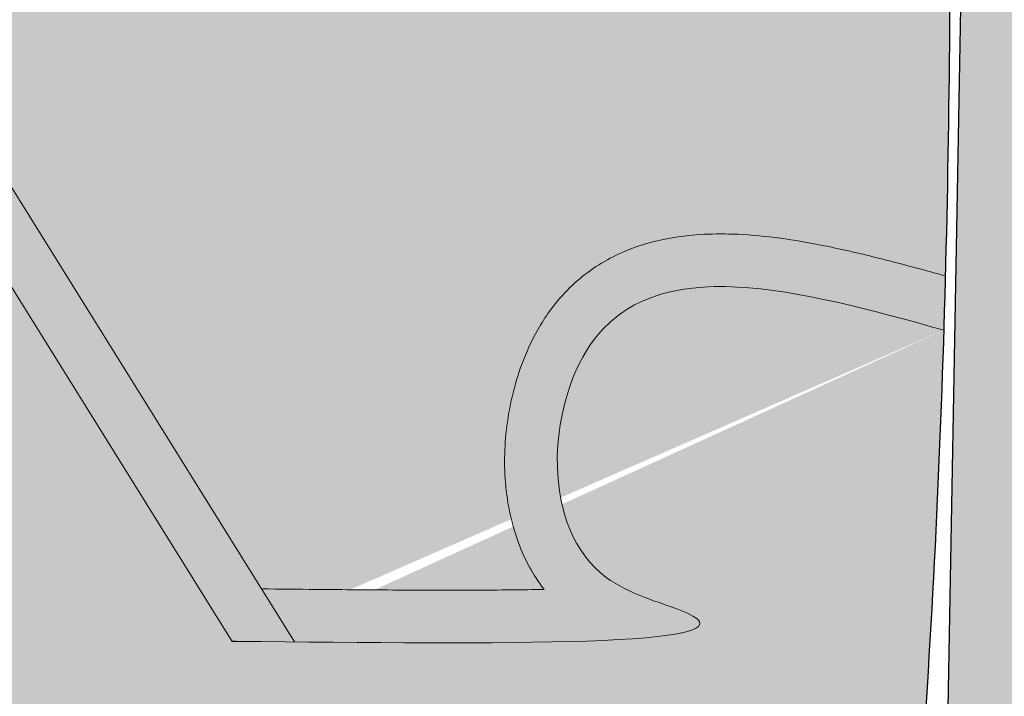
# Model space of a CAD drawing. Units: millimetres. Extents: x 11032 to 26788, y 3406 to 24505.
# Tile 57 of 78: x 16358 to 17293, y 14856 to 15498. Entities that reach past the tile are written whole.
import ezdxf

# ---------------------------------------------------------------- set-up
doc = ezdxf.new("R2010")
doc.units = ezdxf.units.MM
doc.header["$MEASUREMENT"] = 0
for name, color, linetype, lineweight in [('A-ANNO-DIMS', 2, 'Continuous', 18), ('A-ELEV-GUIT', 7, 'Continuous', 18), ('A-GLAZ', 250, 'Continuous', 20), ('A-ROOF', 7, 'Continuous', 30), ('A-WALL', 7, 'Continuous', 35), ('E-LITE', 7, 'Continuous', 18), ('E-LITE-PATT', 7, 'Continuous', 13)]:
    doc.layers.add(name, color=color, linetype=linetype, lineweight=lineweight)
doc.layers.add('A-GLAZ-FRAM-PATT', color=250, linetype='Continuous', lineweight=13, true_color=0x262627)
doc.layers.add('A-ROOF-PATT', color=9, linetype='Continuous', lineweight=13, true_color=0xc7c8ca)
doc.styles.get("Standard").update_dxf_attribs({"font": 'arial.ttf'})
doc.dimstyles.get("Standard").update_dxf_attribs({"dimtxt": 150, "dimasz": 100, "dimexe": 10, "dimexo": 5, "dimgap": 5, "dimtad": 0, "dimtih": 1, "dimtoh": 1, "dimdec": 0, "dimzin": 0, "dimdsep": 46, "dimtxsty": 'Standard', "dimcen": 0.09, "dimadec": 0, "dimazin": 0, "dimtfac": 1, "dimtdec": 0, "dimtofl": 0, "dimtmove": 0, "dimatfit": 3, "dimfxl": 1, "dimtolj": 1, "dimtzin": 0, "dimarcsym": 0})

# ---------------------------------------------------------------- blocks, each defined once
blk = doc.blocks.new('*D36')
at = {"layer": 'A-ANNO-DIMS', "color": 0, "lineweight": -2, "transparency": 16777216}
for p, q in [((12301.26, 17115.89), (12301.26, 24416.86)), ((25397.4, 4466.4), (25397.4, 24416.86)), ((12401.26, 24406.86), (18569.2, 24406.86)), ((25297.4, 24406.86), (19129.47, 24406.86))]:
    blk.add_line(p, q, dxfattribs=at)
at = {"layer": 'A-ANNO-DIMS', "color": 0, "transparency": 16777216}
for points in [[(12401.26, 24423.52), (12401.26, 24390.19), (12301.26, 24406.86)], [(25297.4, 24423.52), (25297.4, 24390.19), (25397.4, 24406.86)]]:
    blk.add_solid(points, dxfattribs=at)
at = {"layer": 'Defpoints', "color": 0, "transparency": 16777216}
for p in [(25397.4, 24406.86), (12301.26, 17110.89), (25397.4, 4461.4)]:
    blk.add_point(p, dxfattribs=at)
at = {"layer": 'A-ANNO-DIMS', "color": 0, "transparency": 16777216, "insert": (18849.33, 24406.86), "char_height": 150, "attachment_point": 5}
blk.add_mtext('\\A1;13096', dxfattribs=at)
blk = doc.blocks.new('*D37')
at = {"layer": 'A-ANNO-DIMS', "color": 0, "lineweight": -2, "transparency": 16777216}
for p, q in [((18087.74, 23450.36), (11334.76, 23450.36)), ((11344.76, 23350.36), (11344.76, 14037.46)), ((11344.76, 4561.4), (11344.76, 13874.29)), ((12927.66, 4461.4), (11334.76, 4461.4))]:
    blk.add_line(p, q, dxfattribs=at)
at = {"layer": 'A-ANNO-DIMS', "color": 0, "transparency": 16777216}
for points in [[(11328.1, 23350.36), (11361.43, 23350.36), (11344.76, 23450.36)], [(11328.1, 4561.4), (11361.43, 4561.4), (11344.76, 4461.4)]]:
    blk.add_solid(points, dxfattribs=at)
at = {"layer": 'Defpoints', "color": 0, "transparency": 16777216}
for p in [(11344.76, 23450.36), (18092.74, 23450.36), (12932.66, 4461.4)]:
    blk.add_point(p, dxfattribs=at)
at = {"layer": 'A-ANNO-DIMS', "color": 0, "transparency": 16777216, "insert": (11344.76, 13955.88), "char_height": 150, "attachment_point": 5}
blk.add_mtext('\\A1;18989', dxfattribs=at)
blk = doc.blocks.new('*D57')
at = {"layer": 'A-ANNO-DIMS', "color": 0, "lineweight": -2, "transparency": 16777216}
for p, q in [((14994.7, 7266.4), (14994.7, 24416.86)), ((20894.7, 7266.4), (20894.7, 24416.86)), ((15094.7, 24406.86), (17715.98, 24406.86)), ((20794.7, 24406.86), (18173.42, 24406.86))]:
    blk.add_line(p, q, dxfattribs=at)
at = {"layer": 'A-ANNO-DIMS', "color": 0, "transparency": 16777216}
for points in [[(15094.7, 24423.52), (15094.7, 24390.19), (14994.7, 24406.86)], [(20794.7, 24423.52), (20794.7, 24390.19), (20894.7, 24406.86)]]:
    blk.add_solid(points, dxfattribs=at)
at = {"layer": 'Defpoints', "color": 0, "transparency": 16777216}
for p in [(20894.7, 24406.86), (14994.7, 7261.4), (20894.7, 7261.4)]:
    blk.add_point(p, dxfattribs=at)
at = {"layer": 'A-ANNO-DIMS', "color": 0, "transparency": 16777216, "insert": (17944.7, 24406.86), "char_height": 150, "attachment_point": 5}
blk.add_mtext('\\A1;5900', dxfattribs=at)

msp = doc.modelspace()

# ---------------------------------------------------------------- hatches: boundary and pattern name
at = {"layer": 'A-GLAZ-FRAM-PATT'}
h = msp.add_hatch(color=256, dxfattribs=at)
edge = h.paths.add_edge_path()
edge.add_line((15784.393, 16248.213), (15784.393, 16153.61))
edge.add_line((15784.393, 16153.61), (16560.042, 14907.752))
edge.add_spline(control_points=[(16560.042, 14907.752), (16569.192, 14907.664), (16578.343, 14907.575), (16587.493, 14907.486), (16598.103, 14907.383), (16608.713, 14907.281), (16619.296, 14907.181)], knot_values=[1012.2878735, 1012.2878735, 1012.2878735, 1012.2878735, 1027.155312, 1027.155312, 1027.155312, 1044.3939449, 1044.3939449, 1044.3939449, 1044.3939449], degree=3, periodic=0)
edge.add_line((16619.296, 14907.181), (15784.393, 16248.213))
at = {"layer": 'A-ROOF-PATT'}
h = msp.add_hatch(color=256, dxfattribs=at)
edge = h.paths.add_edge_path()
edge.add_spline(control_points=[(17532.827, 17324.837), (17391.335, 17349.016), (16840.872, 17494.912), (16080.055, 18069.544), (14738.803, 18299.641), (13382.429, 18838.336), (12580.532, 17870.207), (12430.422, 17563.822)], knot_values=[2977.6027945, 2977.6027945, 2977.6027945, 2977.6027945, 3438.1840601, 4811.6463022, 5622.8675483, 7588.0288188, 8560.6685791, 8560.6685791, 8560.6685791, 8560.6685791], degree=3, periodic=0)
edge.add_spline(control_points=[(12430.422, 17563.822), (12437.904, 17573.36), (12445.386, 17582.899), (12452.869, 17592.437), (12452.869, 17592.438), (12452.869, 17592.438), (12452.869, 17592.438)], knot_values=[1408.564138, 1408.564138, 1408.564138, 1408.564138, 1444.85989, 1444.85989, 1444.85989, 1444.8601183, 1444.8601183, 1444.8601183, 1444.8601183], degree=3, periodic=0)
edge.add_spline(control_points=[(12452.869, 17592.438), (12555.432, 17723.185), (12736.557, 17929.686), (13044.86, 18114.643), (13219.943, 18189.644), (13299.92, 18220.646)], knot_values=[339.318246, 339.318246, 339.318246, 339.318246, 836.8349967, 1151.2512933, 1408.564138, 1408.564138, 1408.564138, 1408.564138], degree=3, periodic=0)
edge.add_spline(control_points=[(13299.92, 18220.646), (13299.998, 18220.689), (13300.077, 18220.732), (13319.738, 18231.488), (13339.24, 18241.402), (13388.645, 18264.703), (13418.466, 18277.069), (13478.019, 18298.648), (13507.751, 18307.861), (13544.561, 18317.488), (13551.584, 18319.245), (13558.612, 18320.924)], knot_values=[3783.8950972, 3783.8950972, 3783.8950972, 3783.8950972, 3784.1737101, 3784.1737101, 3853.4666747, 3853.4666747, 3960.2401917, 3960.2401917, 4067.0137087, 4067.0137087, 4092.1744649, 4092.1744649, 4092.1744649, 4092.1744649], degree=3, periodic=0)
edge.add_spline(control_points=[(13558.612, 18320.924), (13581.407, 18326.373), (13604.25, 18331.007), (13657.184, 18339.957), (13687.338, 18343.732), (13748.098, 18348.892), (13778.704, 18350.276), (13840.46, 18350.833), (13871.609, 18350.005), (13934.496, 18346.313), (13966.232, 18343.449), (14030.297, 18335.871), (14062.625, 18331.158), (14127.853, 18320.088), (14160.753, 18313.73), (14241.357, 18296.556), (14289.343, 18284.997), (14386.31, 18259.688), (14435.291, 18245.941), (14534.161, 18217.034), (14584.049, 18201.875), (14684.682, 18170.964), (14735.427, 18155.212), (14837.763, 18123.971), (14889.354, 18108.482), (14954.971, 18089.677), (14968.586, 18085.823), (14992.391, 18079.184), (15002.566, 18076.376), (15021.739, 18071.153), (15030.731, 18068.729), (15047.707, 18064.21), (15055.694, 18062.106), (15079.815, 18055.825), (15095.905, 18051.728), (15143.966, 18039.717), (15175.729, 18032.084), (15254.84, 18013.501), (15301.798, 18002.866), (15394.186, 17981.845), (15439.615, 17971.459), (15528.833, 17950.135), (15572.62, 17939.197), (15658.477, 17916.021), (15700.546, 17903.785), (15753.633, 17886.734), (15765.446, 17882.835), (15786.574, 17875.653), (15795.915, 17872.404), (15810.108, 17867.349), (15814.99, 17865.588), (15824.736, 17862.029), (15829.611, 17860.226), (15844.241, 17854.75), (15854.002, 17851.008), (15883.312, 17839.521), (15902.885, 17831.512), (15966.355, 17804.548), (16010.39, 17784.302), (16098.838, 17741.267), (16143.25, 17718.478), (16232.497, 17671.098), (16277.332, 17646.507), (16367.515, 17596.295), (16412.862, 17570.676), (16504.202, 17519.209), (16550.194, 17493.362), (16643.009, 17442.263), (16689.831, 17417.011), (16756.517, 17382.472), (16775.937, 17372.58), (16795.455, 17362.84)], knot_values=[4092.1744649, 4092.1744649, 4092.1744649, 4092.1744649, 4173.7872258, 4173.7872258, 4280.5607428, 4280.5607428, 4387.3342598, 4387.3342598, 4494.1077768, 4494.1077768, 4600.8812939, 4600.8812939, 4707.6548109, 4707.6548109, 4814.4283279, 4814.4283279, 4967.1262405, 4967.1262405, 5119.8241531, 5119.8241531, 5272.5220657, 5272.5220657, 5425.2199783, 5425.2199783, 5577.9178908, 5577.9178908, 5617.7853319, 5617.7853319, 5647.4648479, 5647.4648479, 5673.611025, 5673.611025, 5696.747607, 5696.747607, 5743.6818903, 5743.6818903, 5837.5504571, 5837.5504571, 5979.7261046, 5979.7261046, 6121.9017521, 6121.9017521, 6264.0773996, 6264.0773996, 6406.2530471, 6406.2530471, 6447.2585849, 6447.2585849, 6480.0420882, 6480.0420882, 6497.3077062, 6497.3077062, 6514.5733242, 6514.5733242, 6549.1045602, 6549.1045602, 6618.1670322, 6618.1670322, 6772.6610171, 6772.6610171, 6927.155002, 6927.155002, 7081.6489869, 7081.6489869, 7236.1429718, 7236.1429718, 7390.6369567, 7390.6369567, 7545.1309416, 7545.1309416, 7608.1992868, 7608.1992868, 7608.1992868, 7608.1992868], degree=3, periodic=0)
edge.add_spline(control_points=[(16795.455, 17362.84), (16814.335, 17349.456), (16832.897, 17336.263), (16873.225, 17307.197), (16894.778, 17291.386), (16936.221, 17259.941), (16956.11, 17244.308), (16993.863, 17213.094), (17011.726, 17197.514), (17041.993, 17169.265), (17054.791, 17156.601), (17078.762, 17131.225), (17089.933, 17118.516), (17110.618, 17092.991), (17120.131, 17080.178), (17130.17, 17065.264), (17131.487, 17063.277), (17133.77, 17059.776), (17134.746, 17058.261), (17136.69, 17055.205), (17137.657, 17053.668), (17140.539, 17049.025), (17142.438, 17045.89), (17148.068, 17036.367), (17151.732, 17029.859), (17163.03, 17008.788), (17170.335, 16993.646), (17184.087, 16961.978), (17190.534, 16945.453), (17202.562, 16911.165), (17208.142, 16893.402), (17218.448, 16856.821), (17223.173, 16838.003), (17231.801, 16799.51), (17235.705, 16779.837), (17241.533, 16746.739), (17243.676, 16733.5), (17247.718, 16706.37), (17249.608, 16692.472), (17252.066, 16672.69), (17252.761, 16666.875), (17254.1, 16655.226), (17254.744, 16649.4), (17256.596, 16631.917), (17257.727, 16620.254), (17260.823, 16585.238), (17262.489, 16561.858), (17266.551, 16488.654), (17267.658, 16438.661), (17267.349, 16375.228), (17267.193, 16362.07), (17266.95, 16348.891)], knot_values=[15.1130472, 15.1130472, 15.1130472, 15.1130472, 82.6995146, 82.6995146, 165.3990291, 165.3990291, 248.0985437, 248.0985437, 330.7980583, 330.7980583, 397.9419458, 397.9419458, 465.0858333, 465.0858333, 532.2297209, 532.2297209, 542.533741, 542.533741, 550.3568158, 550.3568158, 558.1798906, 558.1798906, 573.8260402, 573.8260402, 605.1183395, 605.1183395, 672.7640614, 672.7640614, 740.4097834, 740.4097834, 808.0555054, 808.0555054, 875.7012273, 875.7012273, 943.3469493, 943.3469493, 987.6613492, 987.6613492, 1033.4121612, 1033.4121612, 1052.3850876, 1052.3850876, 1071.358014, 1071.358014, 1109.3038668, 1109.3038668, 1185.1955724, 1185.1955724, 1346.4419026, 1346.4419026, 1388.5586631, 1388.5586631, 1388.5586631, 1388.5586631], degree=3, periodic=0)
edge.add_spline(control_points=[(17266.95, 16348.891), (17266.95, 16348.891), (17266.95, 16348.891), (17266.95, 16348.891), (17253.182, 15602.417), (17239.414, 14855.943), (17225.646, 14109.469)], knot_values=[1388.5586631, 1388.5586631, 1388.5586631, 1388.5586631, 1388.5589654, 1388.5589654, 1388.5589654, 3774.0767661, 3774.0767661, 3774.0767661, 3774.0767661], degree=3, periodic=0)
edge.add_spline(control_points=[(17225.646, 14109.469), (17226.198, 14109.827), (17226.748, 14110.185), (17242.065, 14120.191), (17255.956, 14130.116), (17274.422, 14144.286), (17279.609, 14148.386), (17284.686, 14152.511)], knot_values=[1926.3423968, 1926.3423968, 1926.3423968, 1926.3423968, 1927.316729, 1927.316729, 1953.5121761, 1953.5121761, 1964.0732348, 1964.0732348, 1964.0732348, 1964.0732348], degree=3, periodic=0)
edge.add_spline(control_points=[(17284.686, 14152.511), (17315.791, 14194.761), (17384.413, 14446.273), (17407.128, 14793.401), (17407.093, 15295.84), (17423.274, 15626.362), (17415.601, 15782.507)], knot_values=[0, 0, 0, 0, 163.2554674, 619.2296767, 1171.8624483, 1621.6355562, 1621.6355562, 1621.6355562, 1621.6355562], degree=3, periodic=0)
edge.add_spline(control_points=[(17415.601, 15782.507), (17438.21, 16077.57), (17410.495, 16533.484), (17390.893, 17030.649), (17301.082, 17169.349)], knot_values=[543.9784753, 543.9784753, 543.9784753, 543.9784753, 1452.9852767, 1960.0114926, 1960.0114926, 1960.0114926, 1960.0114926], degree=3, periodic=0)
edge.add_spline(control_points=[(17301.082, 17169.349), (17346.58, 17157.64), (17392.235, 17147.336), (17467.161, 17132.609), (17496.336, 17127.412), (17525.58, 17122.709)], knot_values=[8131.593939, 8131.593939, 8131.593939, 8131.593939, 8269.7349273, 8269.7349273, 8357.5016646, 8357.5016646, 8357.5016646, 8357.5016646], degree=3, periodic=0)
edge.add_line((17525.58, 17122.709), (17532.827, 17324.837))
edge = h.paths.add_edge_path(flags=17)
edge.add_spline(control_points=[(13340.537, 14602.706), (13316.172, 14726.456), (13323.666, 14932.342), (13637.836, 15081.117), (13863.248, 15171.051), (14002.1, 15224.503), (14058.539, 15244.876)], knot_values=[680.8931862, 680.8931862, 680.8931862, 680.8931862, 1033.4728289, 1337.4008326, 1604.7214264, 1784.2944722, 1784.2944722, 1784.2944722, 1784.2944722], degree=3, periodic=0)
edge.add_spline(control_points=[(14058.539, 15244.876), (14058.289, 15275.236), (14057.634, 15305.434), (14055.312, 15376.527), (14053.359, 15417.248), (14048.642, 15497.048), (14045.89, 15536.143), (14042.888, 15574.619)], knot_values=[6573.1065419, 6573.1065419, 6573.1065419, 6573.1065419, 6636.7330012, 6636.7330012, 6723.8890547, 6723.8890547, 6809.6328771, 6809.6328771, 6809.6328771, 6809.6328771], degree=3, periodic=0)
edge.add_spline(control_points=[(14042.888, 15574.619), (13546.54, 15403.221), (13074.735, 15143.241), (13277.36, 14695.339), (13340.537, 14602.706)], knot_values=[503.7925783, 503.7925783, 503.7925783, 503.7925783, 1728.1787606, 2051.34844, 2051.34844, 2051.34844, 2051.34844], degree=3, periodic=0)
h = msp.add_hatch(color=256, dxfattribs=at)
h.set_gradient(color1=(254, 234, 185), color2=(254, 204, 102), name='HEMISPHERICAL')
edge = h.paths.add_edge_path()
edge.add_spline(control_points=[(16560.042, 14907.752), (16569.192, 14907.664), (16578.343, 14907.575), (16587.493, 14907.486), (16832.101, 14905.115), (17122.895, 14902.296), (16849.359, 14976.117), (16870.954, 15304.114), (17098.337, 15241.178), (17235.385, 15203.245)], knot_values=[0, 0, 0, 0, 14.8674385, 14.8674385, 14.8674385, 412.2943091, 487.3345915, 708.6416004, 1044.3939449, 1044.3939449, 1044.3939449, 1044.3939449], degree=3, periodic=0)
edge.add_line((16587.504, 14907.486), (16560.207, 14907.486))
edge.add_line((16560.207, 14907.486), (15784.393, 16153.61))
edge.add_line((15784.393, 16153.61), (15784.393, 15385.996))
edge.add_spline(control_points=[(15784.393, 15385.996), (15798.391, 15360.52), (15847.198, 15266.214), (15887.196, 15168.614), (15912.903, 15096.727)], knot_values=[1463.2850479, 1463.2850479, 1463.2850479, 1463.2850479, 1550.659771, 1779.9599361, 1779.9599361, 1779.9599361, 1779.9599361], degree=3, periodic=0)
edge.add_spline(control_points=[(15912.903, 15096.727), (15913.652, 15095.649), (15914.403, 15094.565), (15925.191, 15078.948), (15935.516, 15063.47), (15956.582, 15030.918), (15967.324, 15013.844), (15989.119, 14978.386), (16000.173, 14960.003), (16022.525, 14922.193), (16033.824, 14902.767), (16056.63, 14863.116), (16068.138, 14842.891), (16091.349, 14801.871), (16103.053, 14781.075), (16126.666, 14739.118), (16138.575, 14717.958), (16162.628, 14675.459), (16174.772, 14654.12), (16199.352, 14611.428), (16211.787, 14590.075), (16237.037, 14547.491), (16249.851, 14526.26), (16271.946, 14490.566), (16281.092, 14476.044), (16299.694, 14447.129), (16309.149, 14432.737), (16328.456, 14404.098), (16338.307, 14389.85), (16358.518, 14361.503), (16368.879, 14347.403), (16390.266, 14319.347), (16401.291, 14305.391), (16420.626, 14281.969), (16428.703, 14272.467), (16445.363, 14253.527), (16453.946, 14244.088), (16471.727, 14225.278), (16480.926, 14215.907), (16500.075, 14197.247), (16510.026, 14187.959), (16530.844, 14169.504), (16541.71, 14160.337), (16564.549, 14142.195), (16576.522, 14133.22), (16597.69, 14118.448), (16606.528, 14112.565), (16624.87, 14101.004), (16634.376, 14095.326), (16654.117, 14084.255), (16664.352, 14078.862), (16685.603, 14068.46), (16696.619, 14063.452), (16719.46, 14053.944), (16731.285, 14049.444), (16755.742, 14041.097), (16768.374, 14037.251), (16794.396, 14030.368), (16807.787, 14027.332), (16835.229, 14022.23), (16849.279, 14020.163), (16877.882, 14017.141), (16892.435, 14016.186), (16921.835, 14015.489), (16936.683, 14015.749), (16961.564, 14017.241), (16971.582, 14018.127), (16986.57, 14019.883), (16991.56, 14020.54), (16999.027, 14021.63), (17001.514, 14022.011), (17006.48, 14022.809), (17008.962, 14023.225), (17014.824, 14024.251), (17018.193, 14024.875), (17036.262, 14028.398), (17050.55, 14031.826), (17078.171, 14039.583), (17091.505, 14043.912), (17115.643, 14052.705), (17126.557, 14057.089), (17137.108, 14061.688)], knot_values=[2010.7639617, 2010.7639617, 2010.7639617, 2010.7639617, 2014.7029827, 2014.7029827, 2067.238337, 2067.238337, 2119.7736913, 2119.7736913, 2172.3090457, 2172.3090457, 2224.8444, 2224.8444, 2277.3797543, 2277.3797543, 2329.9151086, 2329.9151086, 2382.450463, 2382.450463, 2434.9858173, 2434.9858173, 2487.5211716, 2487.5211716, 2540.0565259, 2540.0565259, 2576.3179289, 2576.3179289, 2612.5793318, 2612.5793318, 2648.8407347, 2648.8407347, 2685.1021376, 2685.1021376, 2721.3635405, 2721.3635405, 2746.252015, 2746.252015, 2771.1404895, 2771.1404895, 2796.028964, 2796.028964, 2820.9174385, 2820.9174385, 2845.8059131, 2845.8059131, 2870.6943876, 2870.6943876, 2887.5132757, 2887.5132757, 2904.3321639, 2904.3321639, 2921.1510521, 2921.1510521, 2937.9699402, 2937.9699402, 2954.7888284, 2954.7888284, 2971.6077166, 2971.6077166, 2988.4266047, 2988.4266047, 3005.2454929, 3005.2454929, 3022.0643811, 3022.0643811, 3038.8832692, 3038.8832692, 3050.1975453, 3050.1975453, 3055.8546833, 3055.8546833, 3058.6832524, 3058.6832524, 3061.5118214, 3061.5118214, 3065.3934173, 3065.3934173, 3082.4668716, 3082.4668716, 3099.5403259, 3099.5403259, 3114.5433443, 3114.5433443, 3114.5433443, 3114.5433443], degree=3, periodic=0)
edge.add_spline(control_points=[(17137.108, 14061.688), (17165.253, 14274.398), (17209.97, 14653.885), (17230.2, 15035.586), (17235.385, 15203.245)], knot_values=[1968.0804557, 1968.0804557, 1968.0804557, 1968.0804557, 2611.5282875, 3114.5379264, 3114.5379264, 3114.5379264, 3114.5379264], degree=3, periodic=0)
edge = h.paths.add_edge_path()
edge.add_spline(control_points=[(16856.103, 14956.992), (16852.841, 14961.219), (16849.83, 14965.576), (16842.539, 14977.287), (16838.658, 14984.798), (16832.033, 15000.109), (16829.289, 15007.911), (16824.126, 15026.008), (16822.047, 15036.354), (16819.308, 15057.097), (16818.649, 15067.496), (16818.576, 15088.188), (16819.162, 15098.483), (16821.467, 15118.823), (16823.186, 15128.868), (16827.696, 15148.567), (16830.486, 15158.22), (16836.065, 15173.969), (16838.565, 15180.211), (16844.079, 15192.402), (16847.092, 15198.353), (16852.029, 15207.021), (16853.744, 15209.868), (16857.321, 15215.468), (16859.188, 15218.226), (16863.017, 15223.558), (16864.978, 15226.136), (16872.565, 15235.558), (16878.593, 15241.952), (16891.428, 15253.591), (16898.232, 15258.834), (16912.397, 15268.127), (16919.756, 15272.176), (16934.816, 15279.138), (16942.515, 15282.052), (16958.1, 15286.873), (16965.985, 15288.78), (16984.013, 15292.142), (16994.186, 15293.334), (17014.631, 15294.619), (17024.904, 15294.713), (17048.453, 15293.935), (17061.76, 15292.783), (17088.519, 15289.422), (17101.972, 15287.211), (17131.961, 15281.46), (17148.526, 15277.734), (17181.692, 15269.627), (17198.292, 15265.245), (17222.182, 15258.759), (17229.535, 15256.737), (17236.862, 15254.714)], knot_values=[9.6639535, 9.6639535, 9.6639535, 9.6639535, 20.0351668, 20.0351668, 36.9411752, 36.9411752, 53.8471837, 53.8471837, 75.7795687, 75.7795687, 97.7119538, 97.7119538, 119.6443388, 119.6443388, 141.5767238, 141.5767238, 163.5091089, 163.5091089, 178.3829945, 178.3829945, 193.2568801, 193.2568801, 200.6938229, 200.6938229, 208.1307657, 208.1307657, 215.4448585, 215.4448585, 235.5795923, 235.5795923, 255.7143261, 255.7143261, 275.8490598, 275.8490598, 295.9837936, 295.9837936, 316.1185274, 316.1185274, 341.7220543, 341.7220543, 367.3255812, 367.3255812, 400.1572431, 400.1572431, 432.988905, 432.988905, 473.0440165, 473.0440165, 513.099128, 513.099128, 530.9692999, 530.9692999, 530.9692999, 530.9692999], degree=3, periodic=0)
edge.add_spline(control_points=[(17236.862, 15254.714), (17240.377, 15387.456), (17242.496, 15609.536), (17239.752, 15831.567), (17250.544, 16044.717)], knot_values=[1250.9818616, 1250.9818616, 1250.9818616, 1250.9818616, 1649.1516581, 1916.613987, 1916.613987, 1916.613987, 1916.613987], degree=3, periodic=0)
edge.add_spline(control_points=[(17250.544, 16044.717), (17229.169, 16066.505), (17207.794, 16088.292), (17186.419, 16110.08), (17186.418, 16110.08), (17186.418, 16110.081), (17186.418, 16110.081)], knot_values=[-88.5185581, -88.5185581, -88.5185581, -88.5185581, -0.0012784, -0.0012784, -0.0012784, 0, 0, 0, 0], degree=3, periodic=0)
edge.add_spline(control_points=[(17186.418, 16110.081), (17169.261, 16127.569), (17151.499, 16145.947), (17114.892, 16184.084), (17096.046, 16203.842), (17057.437, 16244.305), (17037.673, 16265.01), (16997.415, 16306.918), (16976.921, 16328.12), (16927.79, 16378.347), (16898.924, 16407.388), (16840.771, 16464.327), (16811.484, 16492.225), (16758.449, 16540.764), (16734.666, 16561.798), (16687.634, 16601.588), (16664.382, 16620.344), (16624.116, 16650.909), (16606.897, 16663.324), (16583.769, 16678.999), (16577.49, 16683.149), (16567.144, 16689.805), (16563.039, 16692.397), (16550.823, 16699.959), (16542.775, 16704.739), (16526.841, 16713.814), (16518.956, 16718.108), (16495.524, 16730.301), (16480.199, 16737.514), (16449.97, 16750.334), (16435.066, 16755.942), (16405.476, 16765.764), (16390.79, 16769.979), (16361.418, 16777.195), (16346.731, 16780.197), (16317.147, 16785.133), (16302.249, 16787.067), (16272.053, 16789.992), (16256.756, 16790.981), (16225.609, 16792.125), (16209.759, 16792.279), (16177.385, 16791.865), (16160.862, 16791.296), (16136.98, 16790.07), (16129.942, 16789.661), (16118.22, 16788.91), (16113.574, 16788.594), (16103.645, 16787.886), (16098.362, 16787.489), (16087.761, 16786.652), (16082.439, 16786.212), (16066.413, 16784.825), (16055.649, 16783.812), (16023.135, 16780.505), (16001.164, 16777.942), (15934.539, 16769.141), (15889.17, 16761.791), (15797.417, 16743.949), (15751.033, 16733.457), (15645.217, 16705.796), (15585.74, 16687.58), (15526.207, 16666.217), (15525.367, 16665.915), (15524.528, 16665.613)], knot_values=[0, 0, 0, 0, 71.0501454, 71.0501454, 142.1002909, 142.1002909, 213.1504363, 213.1504363, 284.2005818, 284.2005818, 381.323193, 381.323193, 478.4458043, 478.4458043, 557.8219847, 557.8219847, 637.1981651, 637.1981651, 698.3122593, 698.3122593, 721.3971375, 721.3971375, 736.7790891, 736.7790891, 767.5429924, 767.5429924, 798.3068957, 798.3068957, 859.8347022, 859.8347022, 921.3625088, 921.3625088, 982.8903154, 982.8903154, 1044.4181219, 1044.4181219, 1105.9459285, 1105.9459285, 1167.4737351, 1167.4737351, 1229.0015416, 1229.0015416, 1290.5293482, 1290.5293482, 1315.8990035, 1315.8990035, 1332.3812792, 1332.3812792, 1350.9052657, 1350.9052657, 1369.4292522, 1369.4292522, 1406.4772252, 1406.4772252, 1480.5731712, 1480.5731712, 1628.7650633, 1628.7650633, 1776.9569554, 1776.9569554, 1966.3109251, 1966.3109251, 1969.019495, 1969.019495, 1969.019495, 1969.019495], degree=3, periodic=0)
edge.add_line((15524.528, 16665.613), (16587.978, 14957.484))
edge.add_spline(control_points=[(16587.978, 14957.484), (16605.253, 14957.316), (16622.516, 14957.149), (16665.945, 14956.759), (16691.933, 14956.554), (16742.419, 14956.302), (16766.918, 14956.255), (16813.531, 14956.412), (16835.647, 14956.617), (16856.103, 14956.992)], knot_values=[872.2181925, 872.2181925, 872.2181925, 872.2181925, 900.2857301, 900.2857301, 943.3659889, 943.3659889, 986.4462476, 986.4462476, 1029.5265064, 1029.5265064, 1029.5265064, 1029.5265064], degree=3, periodic=0)
h.paths.add_polyline_path([(16474.605, 15622.642, -1), (16624.605, 15622.642, -1)], flags=16)
h.paths.add_polyline_path([(16198.536, 16037.613, -1), (16348.536, 16037.613, -1)], flags=16)
h.paths.add_polyline_path([(16475.717, 16408.125, -1), (16625.717, 16408.125, -1)], flags=16)
at = {"layer": 'E-LITE-PATT'}
h = msp.add_hatch(color=256, dxfattribs=at)
h.paths.add_polyline_path([(13510.178, 17032.97, 1), (13310.178, 17032.97, 1)])
h.paths.add_polyline_path([(14395.599, 17606.181, 1), (14195.599, 17606.181, 1)])
h.paths.add_polyline_path([(16625.717, 16408.125, 1), (16475.717, 16408.125, 1)])
h.paths.add_polyline_path([(16348.536, 16037.613, 1), (16198.536, 16037.613, 1)])
h.paths.add_polyline_path([(16624.605, 15622.642, 1), (16474.605, 15622.642, 1)])
edge = h.paths.add_edge_path()
edge.add_spline(control_points=[(17236.862, 15254.714), (17229.535, 15256.737), (17222.182, 15258.759), (17198.292, 15265.245), (17181.692, 15269.627), (17148.526, 15277.734), (17131.961, 15281.46), (17101.972, 15287.211), (17088.519, 15289.422), (17061.76, 15292.783), (17048.453, 15293.935), (17024.904, 15294.713), (17014.631, 15294.619), (16994.186, 15293.334), (16984.013, 15292.142), (16965.985, 15288.78), (16958.1, 15286.873), (16942.515, 15282.052), (16934.816, 15279.138), (16919.756, 15272.176), (16912.397, 15268.127), (16898.232, 15258.834), (16891.428, 15253.591), (16878.593, 15241.952), (16872.565, 15235.558), (16864.978, 15226.136), (16863.017, 15223.558), (16859.188, 15218.226), (16857.321, 15215.468), (16853.744, 15209.868), (16852.029, 15207.021), (16847.092, 15198.353), (16844.079, 15192.402), (16838.565, 15180.211), (16836.065, 15173.969), (16830.486, 15158.22), (16827.696, 15148.567), (16823.186, 15128.868), (16821.467, 15118.823), (16819.162, 15098.483), (16818.576, 15088.188), (16818.649, 15067.496), (16819.308, 15057.097), (16822.047, 15036.354), (16824.126, 15026.008), (16829.289, 15007.911), (16832.033, 15000.109), (16838.658, 14984.798), (16842.539, 14977.287), (16849.83, 14965.576), (16852.841, 14961.219), (16856.103, 14956.992)], knot_values=[9.6639535, 9.6639535, 9.6639535, 9.6639535, 27.5341253, 27.5341253, 67.5892368, 67.5892368, 107.6443483, 107.6443483, 140.4760102, 140.4760102, 173.3076721, 173.3076721, 198.911199, 198.911199, 224.5147259, 224.5147259, 244.6494597, 244.6494597, 264.7841935, 264.7841935, 284.9189272, 284.9189272, 305.053661, 305.053661, 325.1883948, 325.1883948, 332.5024876, 332.5024876, 339.9394304, 339.9394304, 347.3763732, 347.3763732, 362.2502588, 362.2502588, 377.1241444, 377.1241444, 399.0565295, 399.0565295, 420.9889145, 420.9889145, 442.9212995, 442.9212995, 464.8536846, 464.8536846, 486.7860696, 486.7860696, 503.6920781, 503.6920781, 520.5980866, 520.5980866, 530.9692999, 530.9692999, 530.9692999, 530.9692999], degree=3, periodic=0)
edge.add_spline(control_points=[(16856.103, 14956.992), (16835.647, 14956.617), (16813.531, 14956.412), (16766.918, 14956.255), (16742.419, 14956.302), (16691.933, 14956.554), (16665.945, 14956.759), (16622.516, 14957.149), (16605.253, 14957.316), (16587.978, 14957.484)], knot_values=[872.2181925, 872.2181925, 872.2181925, 872.2181925, 915.2984513, 915.2984513, 958.37871, 958.37871, 1001.4589687, 1001.4589687, 1029.5265064, 1029.5265064, 1029.5265064, 1029.5265064], degree=3, periodic=0)
edge.add_line((16587.978, 14957.484), (16619.296, 14907.181))
edge.add_spline(control_points=[(16619.296, 14907.181), (16852.686, 14904.98), (17116.098, 14904.13), (16849.359, 14976.117), (16870.954, 15304.114), (17098.337, 15241.178), (17235.385, 15203.245)], knot_values=[0, 0, 0, 0, 380.1882376, 455.2285201, 676.535529, 1012.2878735, 1012.2878735, 1012.2878735, 1012.2878735], degree=3, periodic=0)
edge.add_spline(control_points=[(17235.385, 15203.245), (17235.916, 15220.399), (17236.408, 15237.556), (17236.862, 15254.714)], knot_values=[1916.613987, 1916.613987, 1916.613987, 1916.613987, 1968.0804557, 1968.0804557, 1968.0804557, 1968.0804557], degree=3, periodic=0)

# ---------------------------------------------------------------- linework, layer by layer
at = {"layer": 'A-ELEV-GUIT'}
for points, knots in [([(17035.355, 10067.746), (16868.524, 10097.307), (16526.253, 10168.744), (15707.686, 10644.882), (16091.049, 11834.702), (15775.302, 13008.511), (14871.552, 13790.825), (15220.01, 14671.325), (15401.11, 15376.242), (14495.601, 15708.922), (14724.261, 14639.47), (15089.326, 14772.589), (15001.71, 14704.175), (14932.339, 14650.007), (14932.285, 14649.965), (14932.231, 14649.922), (14932.176, 14649.88)], [111.9019878, 111.9019878, 111.9019878, 111.9019878, 624.2629755, 1165.6281599, 2704.5514227, 3555.8315595, 4850.2358438, 5699.326998, 6258.4663613, 6737.7585824, 7501.3569073, 7540.6025682, 7689.8257952, 7689.8257952, 7689.8257952, 7689.9423746, 7689.9423746, 7689.9423746, 7689.9423746]), ([(16985.951, 10051.255), (16959.512, 10056.12), (16933.058, 10061.173), (16828.51, 10082.253), (16750.366, 10100.457), (16653.609, 10129.143), (16634.828, 10134.999), (16597.879, 10147.159), (16579.709, 10153.443), (16548.836, 10164.695), (16536.123, 10169.494), (16510.72, 10179.437), (16498.032, 10184.58), (16460.078, 10200.523), (16434.919, 10211.838), (16365.749, 10245.268), (16322.441, 10268.889), (16239.902, 10320.579), (16200.67, 10348.648), (16136.679, 10402.363), (16110.668, 10427.077), (16080.525, 10460.282), (16074.254, 10467.481), (16060.865, 10483.537), (16053.835, 10492.431), (16040.31, 10510.477), (16033.813, 10519.632), (16015.093, 10547.471), (16003.644, 10566.532), (15976.204, 10617.607), (15961.771, 10650.353), (15937.338, 10717.852), (15927.336, 10752.605), (15911.128, 10823.805), (15904.92, 10860.253), (15895.666, 10934.568), (15892.62, 10972.437), (15888.12, 11070.002), (15888.4, 11130.494), (15892.802, 11253.321), (15896.925, 11315.657), (15906.895, 11441.238), (15912.742, 11504.483), (15924.068, 11630.92), (15929.548, 11694.111), (15938.07, 11819.443), (15941.113, 11881.584), (15942.2, 11964.199), (15942.206, 11985.579), (15941.63, 12024.473), (15941.142, 12042.03), (15939.698, 12076.955), (15938.743, 12094.322), (15935.176, 12146.136), (15931.862, 12180.301), (15919.078, 12281.701), (15906.768, 12347.844), (15874.381, 12477.463), (15854.305, 12540.939), (15806.172, 12665.477), (15778.116, 12726.54), (15738.341, 12800.713), (15730.498, 12814.848), (15715.959, 12840.193), (15709.343, 12851.426), (15695.824, 12873.838), (15688.921, 12885.015), (15667.827, 12918.465), (15653.247, 12940.656), (15608.272, 13006.956), (15576.641, 13050.79), (15511.786, 13138.011), (15478.562, 13181.398), (15412.23, 13268.039), (15379.123, 13311.292), (15314.739, 13398.009), (15283.462, 13441.472), (15224.462, 13528.98), (15196.739, 13573.027), (15146.599, 13662.107), (15124.182, 13707.143), (15090.728, 13788.297), (15078.266, 13824.135), (15064.297, 13875.505), (15060.652, 13890.621), (15054.846, 13918.458), (15052.538, 13931.151), (15049.22, 13952.721), (15048.03, 13961.567), (15045.984, 13979.29), (15045.126, 13988.17), (15043.025, 14014.865), (15042.257, 14032.734), (15041.664, 14088.691), (15043.857, 14127.021), (15052.418, 14204.304), (15058.785, 14243.259), (15074.707, 14321.84), (15084.263, 14361.467), (15105.609, 14441.443), (15117.399, 14481.793), (15148.369, 14583.2), (15168.34, 14644.726), (15193.069, 14722.341), (15197.903, 14737.58), (15206.739, 14765.689), (15210.75, 14778.543), (15217.83, 14801.482), (15220.913, 14811.551), (15226.996, 14831.694), (15229.996, 14841.771), (15238.805, 14871.993), (15244.422, 14892.127), (15257.213, 14941.587), (15263.885, 14970.808), (15274.258, 15028.333), (15277.958, 15056.636), (15280.943, 15105.082), (15281.084, 15125.534), (15278.671, 15165.402), (15276.118, 15184.816), (15268.635, 15219.236), (15264.191, 15234.427), (15252.95, 15263.991), (15246.154, 15278.366), (15229.911, 15306.316), (15220.463, 15319.893), (15198.55, 15346.244), (15185.999, 15359.109), (15158.37, 15383.693), (15143.295, 15395.411), (15111.332, 15417.227), (15094.445, 15427.325), (15059.589, 15445.475), (15041.62, 15453.526), (15005.345, 15467.187), (14987.039, 15472.795), (14950.857, 15481.217), (14932.982, 15484.029), (14902.369, 15486.287), (14889.387, 15486.353), (14864.496, 15484.567), (14852.59, 15482.716), (14832.66, 15477.696), (14824.364, 15474.918), (14808.667, 15468.172), (14801.267, 15464.205), (14791.071, 15457.462), (14787.918, 15455.173), (14782.434, 15450.802), (14780.071, 15448.776), (14775.442, 15444.51), (14773.177, 15442.271), (14766.534, 15435.242), (14762.306, 15430.137), (14754.262, 15419.111), (14750.448, 15413.191), (14741.276, 15397.107), (14736.228, 15386.4), (14727.262, 15363.366), (14723.345, 15351.04), (14716.684, 15325.044), (14713.94, 15311.375), (14709.638, 15282.98), (14708.08, 15268.253), (14705.536, 15228.623), (14705.513, 15203.089), (14708.463, 15151.182), (14711.436, 15124.808), (14720.228, 15072.39), (14726.047, 15046.347), (14740.342, 14995.753), (14748.819, 14971.203), (14768.198, 14924.757), (14779.101, 14902.863), (14799.929, 14868.047), (14809.378, 14854.269), (14829.264, 14829.249), (14839.701, 14818.008), (14858.702, 14800.837), (14867.095, 14794.281), (14884.255, 14782.931), (14893.02, 14778.137), (14910.906, 14770.377), (14920.027, 14767.408), (14938.712, 14763.358), (14948.279, 14762.275), (14968.031, 14762.142), (14978.22, 14763.092), (14991.292, 14765.688), (14993.808, 14766.248), (14999.354, 14767.615), (15002.512, 14768.48), (15008.884, 14770.318), (15012.096, 14771.29), (15017.523, 14772.931), (15019.766, 14773.61), (15023.763, 14774.782), (15025.529, 14775.287), (15028.679, 14776.134), (15030.067, 14776.49), (15032.614, 14777.084), (15033.766, 14777.333), (15035.694, 14777.695), (15036.443, 14777.823), (15038.377, 14778.11), (15039.583, 14778.253), (15042.142, 14778.438), (15043.496, 14778.484), (15046.098, 14778.4), (15047.284, 14778.312), (15049.881, 14777.949), (15051.295, 14777.675), (15053.996, 14776.895), (15055.222, 14776.467), (15057.807, 14775.326), (15059.166, 14774.61), (15061.672, 14772.965), (15062.811, 14772.098), (15065.014, 14770.098), (15066.077, 14768.965), (15068.013, 14766.486), (15068.884, 14765.142), (15070.358, 14762.356), (15070.96, 14760.916), (15071.886, 14758.072), (15072.212, 14756.667), (15072.637, 14753.984), (15072.737, 14752.704), (15072.781, 14750.306), (15072.725, 14749.187), (15072.516, 14747.107), (15072.362, 14746.146), (15071.902, 14743.878), (15071.558, 14742.666), (15070.823, 14740.476), (15070.432, 14739.498), (15069.633, 14737.7), (15069.226, 14736.881), (15068.406, 14735.348), (15067.993, 14734.635), (15066.875, 14732.809), (15066.166, 14731.76), (15064.723, 14729.752), (15063.989, 14728.796), (15062.483, 14726.92), (15061.71, 14726.002), (15059.362, 14723.309), (15057.718, 14721.544), (15054.208, 14717.94), (15052.342, 14716.102), (15048.378, 14712.319), (15046.282, 14710.375), (15039.86, 14704.553), (15035.236, 14700.52), (15025.278, 14692.055), (15019.943, 14687.624), (15008.707, 14678.438), (15002.806, 14673.683), (14988.92, 14662.601), (14980.806, 14656.199), (14972.535, 14649.707)], [157.8567741, 157.8567741, 157.8567741, 157.8567741, 238.7578547, 238.7578547, 477.5157094, 477.5157094, 535.0601182, 535.0601182, 590.8158859, 590.8158859, 629.887765, 629.887765, 668.9596442, 668.9596442, 747.1034024, 747.1034024, 886.5926319, 886.5926319, 1026.0818613, 1026.0818613, 1133.4228819, 1133.4228819, 1162.5976257, 1162.5976257, 1197.5648926, 1197.5648926, 1232.5321594, 1232.5321594, 1302.4666932, 1302.4666932, 1415.5617215, 1415.5617215, 1528.6567499, 1528.6567499, 1641.7517782, 1641.7517782, 1754.8468066, 1754.8468066, 1928.719096, 1928.719096, 2102.5913855, 2102.5913855, 2276.4636749, 2276.4636749, 2450.3359644, 2450.3359644, 2624.2082538, 2624.2082538, 2685.4090323, 2685.4090323, 2736.3317416, 2736.3317416, 2787.2544509, 2787.2544509, 2889.0998694, 2889.0998694, 3092.7907066, 3092.7907066, 3296.4815438, 3296.4815438, 3500.172381, 3500.172381, 3548.3849728, 3548.3849728, 3586.9821961, 3586.9821961, 3625.5794195, 3625.5794195, 3702.7738662, 3702.7738662, 3857.1627597, 3857.1627597, 4011.5516532, 4011.5516532, 4165.9405467, 4165.9405467, 4320.3294401, 4320.3294401, 4474.7183336, 4474.7183336, 4629.1072271, 4629.1072271, 4748.669906, 4748.669906, 4798.1299219, 4798.1299219, 4839.2158308, 4839.2158308, 4867.6081497, 4867.6081497, 4896.0004686, 4896.0004686, 4952.7851064, 4952.7851064, 5073.1303455, 5073.1303455, 5193.4755847, 5193.4755847, 5313.8208238, 5313.8208238, 5434.166063, 5434.166063, 5613.4167284, 5613.4167284, 5657.0185448, 5657.0185448, 5693.5590003, 5693.5590003, 5722.035665, 5722.035665, 5750.5123298, 5750.5123298, 5807.4656593, 5807.4656593, 5891.0584163, 5891.0584163, 5974.6511734, 5974.6511734, 6037.9090774, 6037.9090774, 6101.1669815, 6101.1669815, 6153.5374684, 6153.5374684, 6205.9079554, 6205.9079554, 6258.2784423, 6258.2784423, 6310.6489292, 6310.6489292, 6363.0194161, 6363.0194161, 6415.389903, 6415.389903, 6467.76039, 6467.76039, 6520.1308769, 6520.1308769, 6572.5013638, 6572.5013638, 6612.9787563, 6612.9787563, 6653.4561489, 6653.4561489, 6684.8446676, 6684.8446676, 6716.2331863, 6716.2331863, 6730.9431465, 6730.9431465, 6742.6576959, 6742.6576959, 6754.3722453, 6754.3722453, 6777.8013442, 6777.8013442, 6801.230443, 6801.230443, 6837.5613454, 6837.5613454, 6873.8922478, 6873.8922478, 6910.2231502, 6910.2231502, 6946.5540526, 6946.5540526, 7005.4936024, 7005.4936024, 7064.4331521, 7064.4331521, 7123.3727018, 7123.3727018, 7182.3122516, 7182.3122516, 7241.2518013, 7241.2518013, 7284.9567434, 7284.9567434, 7328.6616855, 7328.6616855, 7361.6324932, 7361.6324932, 7394.603301, 7394.603301, 7427.5741087, 7427.5741087, 7460.5449164, 7460.5449164, 7493.5157242, 7493.5157242, 7501.2914059, 7501.2914059, 7510.5081259, 7510.5081259, 7519.724846, 7519.724846, 7526.3673418, 7526.3673418, 7531.7783017, 7531.7783017, 7536.0875246, 7536.0875246, 7539.5790586, 7539.5790586, 7541.6929901, 7541.6929901, 7544.9601848, 7544.9601848, 7548.2273796, 7548.2273796, 7550.6487832, 7550.6487832, 7553.0701867, 7553.0701867, 7554.8650159, 7554.8650159, 7556.659845, 7556.659845, 7558.1282329, 7558.1282329, 7559.5966208, 7559.5966208, 7561.0650086, 7561.0650086, 7562.5333965, 7562.5333965, 7564.0017844, 7564.0017844, 7565.4701723, 7565.4701723, 7566.9385602, 7566.9385602, 7568.4069481, 7568.4069481, 7570.6698477, 7570.6698477, 7572.9327474, 7572.9327474, 7575.1956471, 7575.1956471, 7577.4585468, 7577.4585468, 7581.2828696, 7581.2828696, 7585.1071924, 7585.1071924, 7588.9315153, 7588.9315153, 7596.3743823, 7596.3743823, 7603.8172493, 7603.8172493, 7611.2601164, 7611.2601164, 7625.457081, 7625.457081, 7639.6540456, 7639.6540456, 7653.8510102, 7653.8510102, 7671.9474465, 7671.9474465, 7671.9474465, 7671.9474465])]:
    msp.add_open_spline(points, degree=3, knots=knots, dxfattribs=at)
at = {"layer": 'A-GLAZ'}
for p, q in [((15284.393, 17051.32), (16619.296, 14907.181)), ((15284.393, 16956.717), (16560.207, 14907.486))]:
    msp.add_line(p, q, dxfattribs=at)
at = {"layer": 'A-ROOF'}
for points, knots in [([(16795.455, 17362.84), (16814.335, 17349.456), (16832.897, 17336.263), (16873.225, 17307.197), (16894.778, 17291.386), (16936.221, 17259.941), (16956.11, 17244.308), (16993.863, 17213.094), (17011.726, 17197.514), (17041.993, 17169.265), (17054.791, 17156.601), (17078.762, 17131.225), (17089.933, 17118.516), (17110.618, 17092.991), (17120.131, 17080.178), (17130.17, 17065.264), (17131.487, 17063.277), (17133.77, 17059.776), (17134.746, 17058.261), (17136.69, 17055.205), (17137.657, 17053.668), (17140.539, 17049.025), (17142.438, 17045.89), (17148.068, 17036.367), (17151.732, 17029.859), (17163.03, 17008.788), (17170.335, 16993.646), (17184.087, 16961.978), (17190.534, 16945.453), (17202.562, 16911.165), (17208.142, 16893.402), (17218.448, 16856.821), (17223.173, 16838.003), (17231.801, 16799.51), (17235.705, 16779.837), (17241.533, 16746.739), (17243.676, 16733.5), (17247.718, 16706.37), (17249.608, 16692.472), (17252.066, 16672.69), (17252.761, 16666.875), (17254.1, 16655.226), (17254.744, 16649.4), (17256.596, 16631.917), (17257.727, 16620.254), (17260.823, 16585.238), (17262.489, 16561.858), (17266.551, 16488.654), (17267.658, 16438.661), (17267.349, 16375.228), (17267.193, 16362.07), (17266.95, 16348.891), (17266.95, 16348.891), (17266.95, 16348.891), (17266.95, 16348.891), (17253.182, 15602.417), (17239.414, 14855.943), (17225.646, 14109.469)], [15.1130472, 15.1130472, 15.1130472, 15.1130472, 82.6995146, 82.6995146, 165.3990291, 165.3990291, 248.0985437, 248.0985437, 330.7980583, 330.7980583, 397.9419458, 397.9419458, 465.0858333, 465.0858333, 532.2297209, 532.2297209, 542.533741, 542.533741, 550.3568158, 550.3568158, 558.1798906, 558.1798906, 573.8260402, 573.8260402, 605.1183395, 605.1183395, 672.7640614, 672.7640614, 740.4097834, 740.4097834, 808.0555054, 808.0555054, 875.7012273, 875.7012273, 943.3469493, 943.3469493, 987.6613492, 987.6613492, 1033.4121612, 1033.4121612, 1052.3850876, 1052.3850876, 1071.358014, 1071.358014, 1109.3038668, 1109.3038668, 1185.1955724, 1185.1955724, 1346.4419026, 1346.4419026, 1388.5586631, 1388.5586631, 1388.5586631, 1388.5589654, 1388.5589654, 1388.5589654, 3774.0767661, 3774.0767661, 3774.0767661, 3774.0767661]), ([(17266.95, 16348.891), (17262.307, 16263.231), (17257.663, 16177.571), (17253.02, 16091.911), (17253.019, 16091.901), (17253.019, 16091.892), (17253.018, 16091.882), (17239.592, 15844.196), (17244.957, 15430.9), (17227.508, 14802.718), (17165.253, 14274.398), (17137.108, 14061.688)], [1132.9967717, 1132.9967717, 1132.9967717, 1132.9967717, 1232.0405278, 1232.0405278, 1232.0405278, 1232.05171, 1232.05171, 1232.05171, 1518.4441905, 2471.0900946, 3114.5379264, 3114.5379264, 3114.5379264, 3114.5379264])]:
    msp.add_open_spline(points, degree=3, knots=knots, dxfattribs=at)
at = {"layer": 'A-WALL'}
for points, knots in [([(17415.601, 15782.507), (17423.274, 15626.362), (17407.093, 15295.84), (17407.128, 14793.401), (17384.413, 14446.273), (17315.791, 14194.761), (17284.686, 14152.511)], [0, 0, 0, 0, 449.7731079, 1002.4058796, 1458.3800888, 1621.6355562, 1621.6355562, 1621.6355562, 1621.6355562]), ([(17284.686, 14152.511), (17279.609, 14148.386), (17274.422, 14144.286), (17255.956, 14130.116), (17242.065, 14120.191), (17215.521, 14102.851), (17203.187, 14095.335), (17177.254, 14080.821), (17163.654, 14073.822), (17135.064, 14060.571), (17120.072, 14054.319), (17091.505, 14043.912), (17078.171, 14039.583), (17050.55, 14031.826), (17036.262, 14028.398), (17018.193, 14024.875), (17014.824, 14024.251), (17008.962, 14023.225), (17006.48, 14022.809), (17001.514, 14022.011), (16999.027, 14021.63), (16991.56, 14020.54), (16986.57, 14019.883), (16971.582, 14018.127), (16961.564, 14017.241), (16936.683, 14015.749), (16921.835, 14015.489), (16892.435, 14016.186), (16877.882, 14017.141), (16849.279, 14020.163), (16835.229, 14022.23), (16807.787, 14027.332), (16794.396, 14030.368), (16768.374, 14037.251), (16755.742, 14041.097), (16731.285, 14049.444), (16719.46, 14053.944), (16696.619, 14063.452), (16685.603, 14068.46), (16664.352, 14078.862), (16654.117, 14084.255), (16634.376, 14095.326), (16624.87, 14101.004), (16606.528, 14112.565), (16597.69, 14118.448), (16576.522, 14133.22), (16564.549, 14142.195), (16541.71, 14160.337), (16530.844, 14169.504), (16510.026, 14187.959), (16500.075, 14197.247), (16480.926, 14215.907), (16471.727, 14225.278), (16453.946, 14244.088), (16445.363, 14253.527), (16428.703, 14272.467), (16420.626, 14281.969), (16401.291, 14305.391), (16390.266, 14319.347), (16368.879, 14347.403), (16358.518, 14361.503), (16338.307, 14389.85), (16328.456, 14404.098), (16309.149, 14432.737), (16299.694, 14447.129), (16281.092, 14476.044), (16271.946, 14490.566), (16249.851, 14526.26), (16237.037, 14547.491), (16211.787, 14590.075), (16199.352, 14611.428), (16174.772, 14654.12), (16162.628, 14675.459), (16138.575, 14717.958), (16126.666, 14739.118), (16103.053, 14781.075), (16091.349, 14801.871), (16068.138, 14842.891), (16056.63, 14863.116), (16033.824, 14902.767), (16022.525, 14922.193), (16000.173, 14960.003), (15989.119, 14978.386), (15967.324, 15013.844), (15956.582, 15030.918), (15935.516, 15063.47), (15925.191, 15078.948), (15914.403, 15094.565), (15913.652, 15095.649), (15912.903, 15096.727)], [1926.3423968, 1926.3423968, 1926.3423968, 1926.3423968, 1936.9034555, 1936.9034555, 1963.0989026, 1963.0989026, 1983.9882618, 1983.9882618, 2004.8776209, 2004.8776209, 2025.7669801, 2025.7669801, 2042.8404344, 2042.8404344, 2059.9138887, 2059.9138887, 2063.7954846, 2063.7954846, 2066.6240536, 2066.6240536, 2069.4526227, 2069.4526227, 2075.1097607, 2075.1097607, 2086.4240368, 2086.4240368, 2103.2429249, 2103.2429249, 2120.0618131, 2120.0618131, 2136.8807013, 2136.8807013, 2153.6995894, 2153.6995894, 2170.5184776, 2170.5184776, 2187.3373658, 2187.3373658, 2204.1562539, 2204.1562539, 2220.9751421, 2220.9751421, 2237.7940303, 2237.7940303, 2254.6129184, 2254.6129184, 2279.5013929, 2279.5013929, 2304.3898675, 2304.3898675, 2329.278342, 2329.278342, 2354.1668165, 2354.1668165, 2379.055291, 2379.055291, 2403.9437655, 2403.9437655, 2440.2051684, 2440.2051684, 2476.4665713, 2476.4665713, 2512.7279742, 2512.7279742, 2548.9893772, 2548.9893772, 2585.2507801, 2585.2507801, 2637.7861344, 2637.7861344, 2690.3214887, 2690.3214887, 2742.856843, 2742.856843, 2795.3921974, 2795.3921974, 2847.9275517, 2847.9275517, 2900.462906, 2900.462906, 2952.9982603, 2952.9982603, 3005.5336147, 3005.5336147, 3058.068969, 3058.068969, 3110.6043233, 3110.6043233, 3114.5433443, 3114.5433443, 3114.5433443, 3114.5433443])]:
    msp.add_open_spline(points, degree=3, knots=knots, dxfattribs=at)
at = {"layer": 'E-LITE'}
msp.add_line((16587.493, 14907.486), (16560.207, 14907.486), dxfattribs=at)
for points, knots in [([(17236.862, 15254.714), (17229.535, 15256.737), (17222.182, 15258.759), (17198.292, 15265.245), (17181.692, 15269.627), (17148.526, 15277.734), (17131.961, 15281.46), (17101.972, 15287.211), (17088.519, 15289.422), (17061.76, 15292.783), (17048.453, 15293.935), (17024.904, 15294.713), (17014.631, 15294.619), (16994.186, 15293.334), (16984.013, 15292.142), (16965.985, 15288.78), (16958.1, 15286.873), (16942.515, 15282.052), (16934.816, 15279.138), (16919.756, 15272.176), (16912.397, 15268.127), (16898.232, 15258.834), (16891.428, 15253.591), (16878.593, 15241.952), (16872.565, 15235.558), (16864.978, 15226.136), (16863.017, 15223.558), (16859.188, 15218.226), (16857.321, 15215.468), (16853.744, 15209.868), (16852.029, 15207.021), (16847.092, 15198.353), (16844.079, 15192.402), (16838.565, 15180.211), (16836.065, 15173.969), (16830.486, 15158.22), (16827.696, 15148.567), (16823.186, 15128.868), (16821.467, 15118.823), (16819.162, 15098.483), (16818.576, 15088.188), (16818.649, 15067.496), (16819.308, 15057.097), (16822.047, 15036.354), (16824.126, 15026.008), (16829.289, 15007.911), (16832.033, 15000.109), (16838.658, 14984.798), (16842.539, 14977.287), (16849.83, 14965.576), (16852.841, 14961.219), (16856.103, 14956.992)], [9.6639535, 9.6639535, 9.6639535, 9.6639535, 27.5341253, 27.5341253, 67.5892368, 67.5892368, 107.6443483, 107.6443483, 140.4760102, 140.4760102, 173.3076721, 173.3076721, 198.911199, 198.911199, 224.5147259, 224.5147259, 244.6494597, 244.6494597, 264.7841935, 264.7841935, 284.9189272, 284.9189272, 305.053661, 305.053661, 325.1883948, 325.1883948, 332.5024876, 332.5024876, 339.9394304, 339.9394304, 347.3763732, 347.3763732, 362.2502588, 362.2502588, 377.1241444, 377.1241444, 399.0565295, 399.0565295, 420.9889145, 420.9889145, 442.9212995, 442.9212995, 464.8536846, 464.8536846, 486.7860696, 486.7860696, 503.6920781, 503.6920781, 520.5980866, 520.5980866, 530.9692999, 530.9692999, 530.9692999, 530.9692999]), ([(17235.385, 15203.245), (17098.337, 15241.178), (16870.954, 15304.114), (16849.359, 14976.117), (17122.895, 14902.296), (16832.101, 14905.115), (16587.493, 14907.486), (16578.343, 14907.575), (16569.192, 14907.664), (16560.042, 14907.752)], [0, 0, 0, 0, 335.7523445, 557.0593534, 632.0996358, 1029.5265064, 1029.5265064, 1029.5265064, 1044.3939449, 1044.3939449, 1044.3939449, 1044.3939449]), ([(16856.103, 14956.992), (16835.647, 14956.617), (16813.531, 14956.412), (16766.918, 14956.255), (16742.419, 14956.302), (16691.933, 14956.554), (16665.945, 14956.759), (16622.516, 14957.149), (16605.253, 14957.316), (16587.978, 14957.484)], [872.2181925, 872.2181925, 872.2181925, 872.2181925, 915.2984513, 915.2984513, 958.37871, 958.37871, 1001.4589687, 1001.4589687, 1029.5265064, 1029.5265064, 1029.5265064, 1029.5265064])]:
    msp.add_open_spline(points, degree=3, knots=knots, dxfattribs=at)

# ---------------------------------------------------------------- dimensions: what is measured, and where the dimension line sits
at = {"layer": 'A-ANNO-DIMS'}
for base, p1, p2, picture, middle in [((25397.404, 24406.858), (12301.265, 17110.885), (25397.404, 4461.399), '*D36', (18849.334, 24406.858)), ((20894.704, 24406.858), (14994.704, 7261.399), (20894.704, 7261.399), '*D57', (17944.704, 24406.858))]:
    dim = msp.add_linear_dim(base=base, p1=p1, p2=p2, dimstyle='Standard', override={"dimdec": 0, "dimlfac": 1, "dimrnd": 0, "dimzin": 0, "dimdsep": 46, "dimlunit": 2}, dxfattribs=at)
    dim.commit()
    dim.dimension.update_dxf_attribs({"geometry": picture, "text_midpoint": middle})
dim = msp.add_linear_dim(base=(11344.765, 23450.358), p1=(12932.665, 4461.399), p2=(18092.739, 23450.358), angle=90, dimstyle='Standard', override={"dimdec": 0, "dimlfac": 1, "dimrnd": 0, "dimzin": 0, "dimdsep": 46, "dimlunit": 2}, dxfattribs=at)
dim.commit()
dim.dimension.update_dxf_attribs({"geometry": '*D37', "text_midpoint": (11344.765, 13955.879)})

doc.saveas('drawing.dxf')
